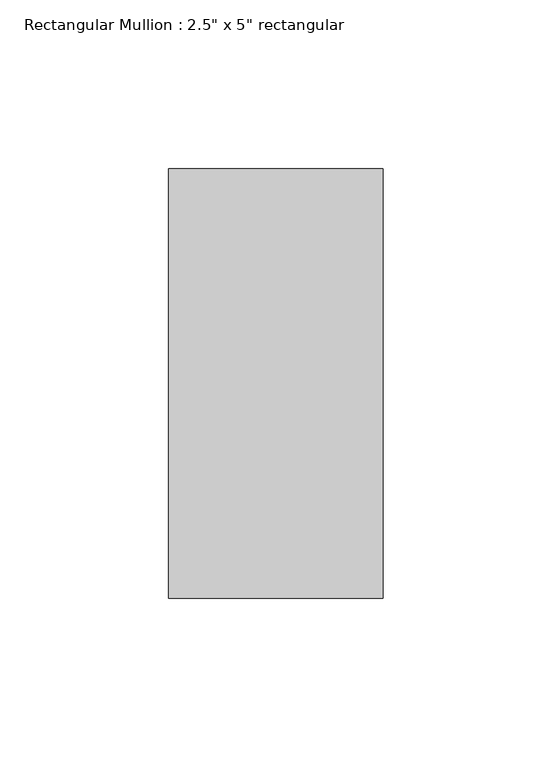
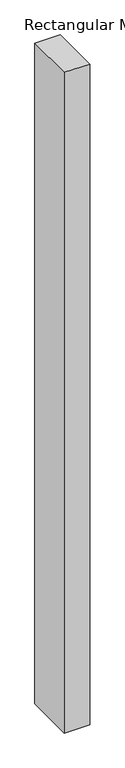
"""IFC4 building model written with IfcOpenShell, lengths in millimetres: member geometry."""

from ifc_helpers import new_model, si_unit, frame, origin, place, context, project, spatial, polyline, outline, extrude, source, transform, mapped, element, save


def member_273748f4(model_context):
    return source(origin(), model_context, "Body", "SweptSolid", [
        extrude(outline(polyline([(0.0, 63.5), (0.0, -63.5), (-63.5, -63.5), (-63.5, 63.5), (0.0, 63.5)])), frame((0.0, 0.0, -1744.0799136), z_axis=(0.0, 0.0, 1.0), x_axis=(1.0, 0.0, 0.0)), (0.0, 0.0, 1.0), 1744.0799136),
    ])


if __name__ == "__main__":
    model = new_model("IFC4")
    model_context = context("Model", 3, world=origin())
    ifc_project = project(units=[si_unit("LENGTHUNIT", "METRE", prefix="MILLI")], contexts=[model_context])
    site = spatial("IfcSite", under=ifc_project)
    building = spatial("IfcBuilding", under=site)
    placement = place(None, origin())
    member_shape = member_273748f4(model_context)
    element("IfcMember", 1, ObjectType="Rectangular Mullion : 2.5\" x 5\" rectangular", at=placement, inside=building, context=model_context, shape_type="MappedRepresentation", body=[
        mapped(member_shape, transform((0.0, 0.0, 0.0), x_axis=(1.0, 0.0, 0.0), y_axis=(0.0, 1.0, 0.0), z_axis=(0.0, 0.0, 1.0))),
    ])
    save(model, "model.ifc")

# Revit data of these elements
# Type "Rectangular Mullion : 2.5\" x 5\" rectangular"
#   built-in parameter 1007304 = 0.416667 (stored number, unit not read)
#   built-in parameter 1007301 = 0.104167 (stored number, unit not read)
#   built-in parameter 1007300 = 0.104167 (stored number, unit not read)
# Element 1 (IfcMember, "Rectangular Mullion : 2.5\" x 5\" rectangular")
#   Materials on its faces: "Aluminum"
# Materials
#   "Aluminum": class "Metal", colour RGB 247 247 247, transparency 0, Description = "Aluminum 6061", Cost = 0
